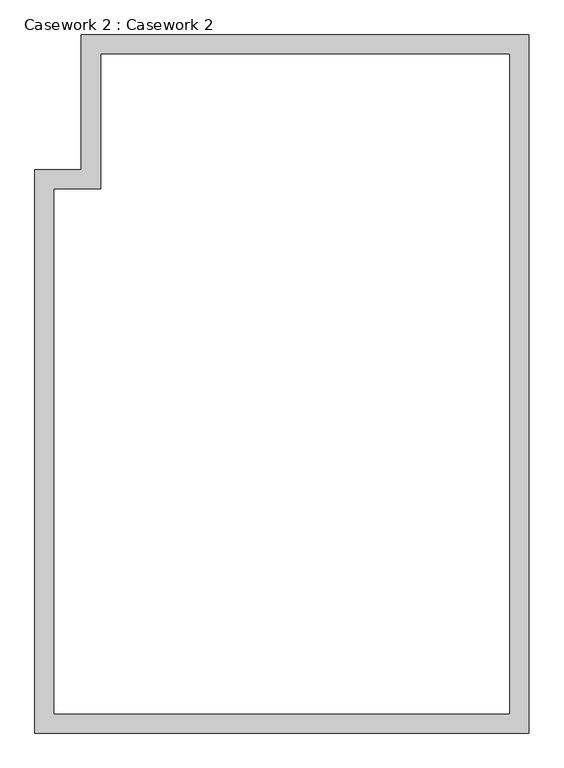
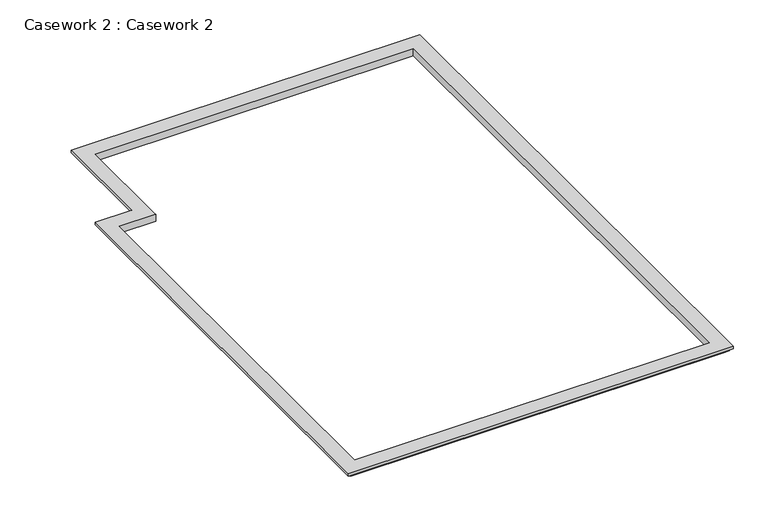
"""IFC4 building model written with IfcOpenShell, lengths in millimetres: furniture geometry, Casework 2 : Casework 2."""

from ifc_helpers import new_model, si_unit, origin, place, context, project, spatial, faceted_brep, source, transform, mapped, element, save


def casework_2_casework_2_b6b509d5(model_context):
    return source(origin(), model_context, "Body", "Brep", [
        faceted_brep([(7838.2046034, 9090.8070837, 3750.0), (7838.2046034, 9090.8070837, 4050.0), (-4686.7953966, 9090.8070837, 4050.0), (-4686.7953966, 9090.8070837, 3750.0), (8238.2046034, 9490.8070837, 3850.0), (8238.2046034, 9490.8070837, 3750.0), (-5086.7953966, 9490.8070837, 3750.0), (-5086.7953966, 9490.8070837, 3850.0), (8338.2046034, 9590.8070837, 3950.0), (8338.2046034, 9590.8070837, 3850.0), (-5186.7953966, 9590.8070837, 3850.0), (-5186.7953966, 9590.8070837, 3950.0), (8438.2046034, 9690.8070837, 4050.0), (8438.2046034, 9690.8070837, 3950.0), (-5286.7953966, 9690.8070837, 3950.0), (-5286.7953966, 9690.8070837, 4050.0), (-4686.7953966, 4965.8070837, 4050.0), (-4686.7953966, 4965.8070837, 3750.0), (-5086.7953966, 5365.8070837, 3750.0), (-5086.7953966, 5365.8070837, 3850.0), (-5186.7953966, 5465.8070837, 3850.0), (-5186.7953966, 5465.8070837, 3950.0), (-5286.7953966, 5565.8070837, 3950.0), (-5286.7953966, 5565.8070837, 4050.0), (-6111.7953966, 4965.8070837, 4050.0), (-6111.7953966, 4965.8070837, 3750.0), (-6511.7953966, 5365.8070837, 3750.0), (-6511.7953966, 5365.8070837, 3850.0), (-6611.7953966, 5465.8070837, 3850.0), (-6611.7953966, 5465.8070837, 3950.0), (-6711.7953966, 5565.8070837, 3950.0), (-6711.7953966, 5565.8070837, 4050.0), (-6111.7953966, -11096.6929163, 4050.0), (-6111.7953966, -11096.6929163, 3750.0), (-6511.7953966, -11496.6929163, 3750.0), (-6511.7953966, -11496.6929163, 3850.0), (-6611.7953966, -11596.6929163, 3850.0), (-6611.7953966, -11596.6929163, 3950.0), (-6711.7953966, -11696.6929163, 3950.0), (-6711.7953966, -11696.6929163, 4050.0), (7838.2046034, -11096.6929163, 4050.0), (7838.2046034, -11096.6929163, 3750.0), (8238.2046034, -11496.6929163, 3750.0), (8238.2046034, -11496.6929163, 3850.0), (8338.2046034, -11596.6929163, 3850.0), (8338.2046034, -11596.6929163, 3950.0), (8438.2046034, -11696.6929163, 3950.0), (8438.2046034, -11696.6929163, 4050.0)], [[[0, 1, 2, 3]], [[4, 5, 6, 7]], [[8, 9, 10, 11]], [[12, 13, 14, 15]], [[3, 2, 16, 17]], [[7, 6, 18, 19]], [[11, 10, 20, 21]], [[15, 14, 22, 23]], [[17, 16, 24, 25]], [[19, 18, 26, 27]], [[21, 20, 28, 29]], [[23, 22, 30, 31]], [[25, 24, 32, 33]], [[27, 26, 34, 35]], [[29, 28, 36, 37]], [[31, 30, 38, 39]], [[33, 32, 40, 41]], [[35, 34, 42, 43]], [[37, 36, 44, 45]], [[39, 38, 46, 47]], [[41, 40, 1, 0]], [[43, 42, 5, 4]], [[45, 44, 9, 8]], [[47, 46, 13, 12]], [[39, 47, 12, 15, 23, 31], [2, 1, 40, 32, 24, 16]], [[6, 5, 42, 34, 26, 18], [33, 41, 0, 3, 17, 25]], [[10, 9, 44, 36, 28, 20], [35, 43, 4, 7, 19, 27]], [[14, 13, 46, 38, 30, 22], [37, 45, 8, 11, 21, 29]]]),
    ])


if __name__ == "__main__":
    model = new_model("IFC4")
    model_context = context("Model", 3, world=origin())
    ifc_project = project(units=[si_unit("LENGTHUNIT", "METRE", prefix="MILLI")], contexts=[model_context])
    site = spatial("IfcSite", under=ifc_project)
    building = spatial("IfcBuilding", under=site)
    placement = place(None, origin())
    casework_2_casework_2_shape = casework_2_casework_2_b6b509d5(model_context)
    element("IfcFurniture", 1, ObjectType="Casework 2 : Casework 2", at=placement, inside=building, context=model_context, shape_type="MappedRepresentation", body=[
        mapped(casework_2_casework_2_shape, transform((0.0, 0.0, 0.0), x_axis=(1.0, 0.0, 0.0), y_axis=(0.0, 1.0, 0.0), z_axis=(0.0, 0.0, 1.0))),
    ])
    save(model, "model.ifc")
